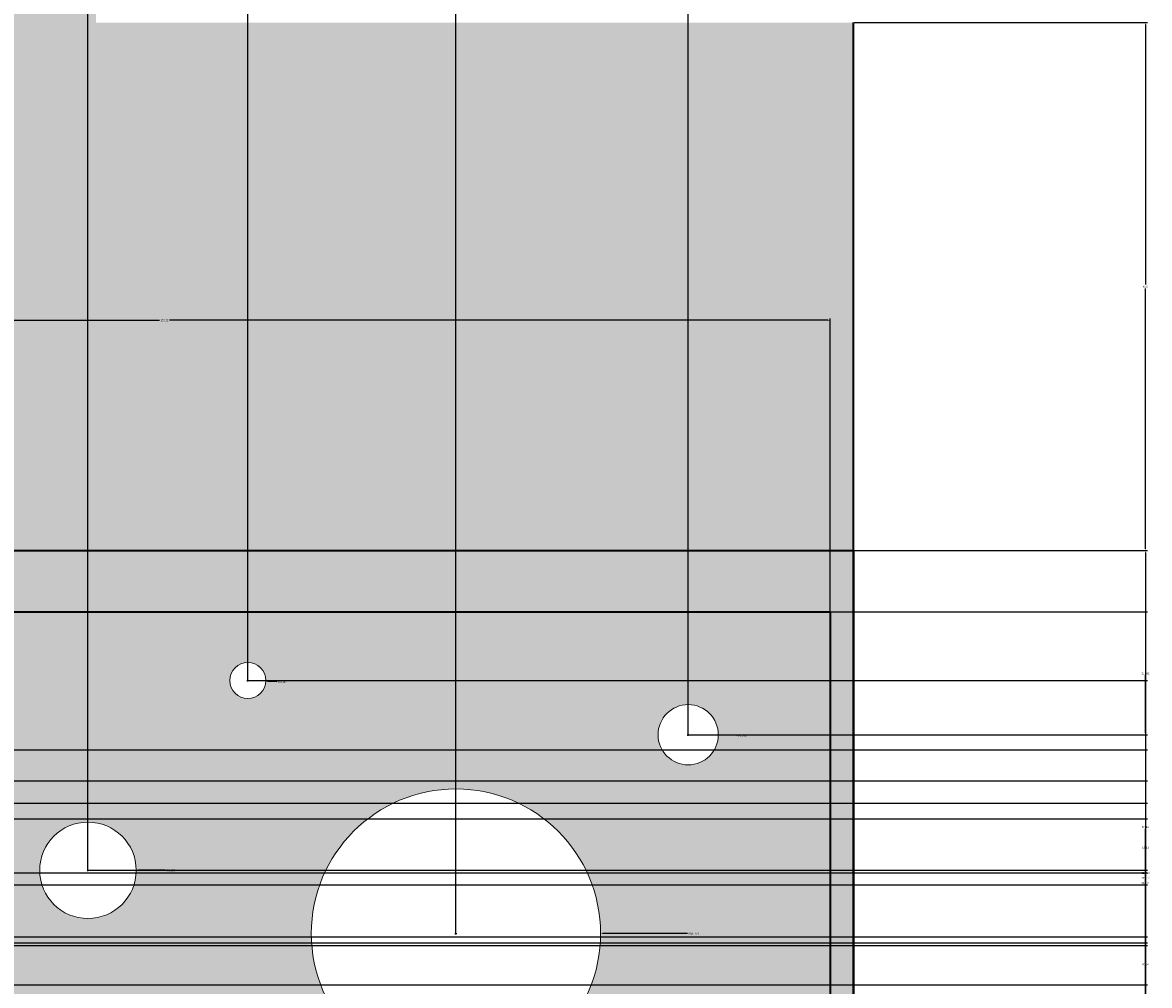
# Model space of a CAD drawing. Units: inches. Extents: x 73 to 607, y 92 to 651.
# Tile 12 of 18: x 503 to 607, y 222 to 311. Entities that reach past the tile are written whole.
import ezdxf

# ---------------------------------------------------------------- set-up
doc = ezdxf.new("R2010")
doc.units = ezdxf.units.IN
doc.header["$MEASUREMENT"] = 0
for name, color, linetype, lineweight in [('A-ANNO-DIMS', 2, 'Continuous', 18), ('A-ELEV', 7, 'Continuous', 35), ('A-ELEV-PANL', 7, 'Continuous', 18), ('A-ELEV-PATT-BKGD', 252, 'Continuous', 13), ('A-ELEV-PATT-SHAD', 8, 'Continuous', 13), ('A-ELEV-PATT-WALL', 254, 'Continuous', 13), ('A-ELEV-PATT-WOOD', 32, 'Continuous', 13)]:
    doc.layers.add(name, color=color, linetype=linetype, lineweight=lineweight)
doc.styles.get("Standard").update_dxf_attribs({"font": 'arial.ttf'})
doc.dimstyles.get("Standard").update_dxf_attribs({"dimtxt": 0.18, "dimasz": 0.18, "dimexe": 0.18, "dimexo": 0.0625, "dimgap": 0.09, "dimtad": 0, "dimtih": 1, "dimtoh": 1, "dimdec": 4, "dimzin": 0, "dimdsep": 46, "dimtxsty": 'Standard', "dimcen": 0.09, "dimadec": 0, "dimazin": 0, "dimtfac": 1, "dimtdec": 4, "dimtofl": 0, "dimtmove": 0, "dimatfit": 3, "dimfxl": 1, "dimtolj": 1, "dimtzin": 0, "dimarcsym": 0})

# ---------------------------------------------------------------- blocks, each defined once
blk = doc.blocks.new('*D17')
at = {"layer": 'A-ANNO-DIMS', "color": 0, "lineweight": -2, "transparency": 16777216}
for p, q in [((580.16, 262.3), (607.28, 262.3)), ((607.1, 262.12), (607.1, 224.16)), ((607.1, 185.84), (607.1, 223.8)), ((431.13, 185.66), (607.28, 185.66))]:
    blk.add_line(p, q, dxfattribs=at)
at = {"layer": 'A-ANNO-DIMS', "color": 0, "transparency": 16777216}
for points in [[(607.07, 262.12), (607.13, 262.12), (607.1, 262.3)], [(607.07, 185.84), (607.13, 185.84), (607.1, 185.66)]]:
    blk.add_solid(points, dxfattribs=at)
at = {"layer": 'Defpoints', "color": 0, "transparency": 16777216}
for p in [(580.1, 262.3), (607.1, 262.3), (431.07, 185.66)]:
    blk.add_point(p, dxfattribs=at)
at = {"layer": 'A-ANNO-DIMS', "color": 0, "transparency": 16777216, "insert": (607.1, 223.98), "char_height": 0.18, "attachment_point": 5}
blk.add_mtext('\\A1;76.64', dxfattribs=at)
blk = doc.blocks.new('*D18')
at = {"layer": 'A-ANNO-DIMS', "color": 0, "lineweight": -2, "transparency": 16777216}
for p, q in [((580.16, 311.2), (607.28, 311.2)), ((607.1, 311.02), (607.1, 286.94)), ((607.1, 262.48), (607.1, 286.57)), ((580.16, 262.3), (607.28, 262.3))]:
    blk.add_line(p, q, dxfattribs=at)
at = {"layer": 'A-ANNO-DIMS', "color": 0, "transparency": 16777216}
for points in [[(607.07, 311.02), (607.13, 311.02), (607.1, 311.2)], [(607.07, 262.48), (607.13, 262.48), (607.1, 262.3)]]:
    blk.add_solid(points, dxfattribs=at)
at = {"layer": 'Defpoints', "color": 0, "transparency": 16777216}
for p in [(580.1, 311.2), (607.1, 311.2), (580.1, 262.3)]:
    blk.add_point(p, dxfattribs=at)
at = {"layer": 'A-ANNO-DIMS', "color": 0, "transparency": 16777216, "insert": (607.1, 286.75), "char_height": 0.18, "attachment_point": 5}
blk.add_mtext('\\A1;48.9', dxfattribs=at)
blk = doc.blocks.new('*D39')
at = {"layer": 'A-ANNO-DIMS', "color": 0, "lineweight": -2, "transparency": 16777216}
for p, q in [((454.7, 256.69), (454.7, 283.81)), ((577.92, 256.69), (577.92, 283.81)), ((454.88, 283.63), (515.86, 283.63)), ((577.74, 283.63), (516.77, 283.63))]:
    blk.add_line(p, q, dxfattribs=at)
at = {"layer": 'A-ANNO-DIMS', "color": 0, "transparency": 16777216}
for points in [[(454.88, 283.66), (454.88, 283.6), (454.7, 283.63)], [(577.74, 283.66), (577.74, 283.6), (577.92, 283.63)]]:
    blk.add_solid(points, dxfattribs=at)
at = {"layer": 'Defpoints', "color": 0, "transparency": 16777216}
for p in [(577.92, 283.63), (454.7, 256.63), (577.92, 256.63)]:
    blk.add_point(p, dxfattribs=at)
at = {"layer": 'A-ANNO-DIMS', "color": 0, "transparency": 16777216, "insert": (516.31, 283.63), "char_height": 0.18, "attachment_point": 5}
blk.add_mtext('\\A1;123.22', dxfattribs=at)
blk = doc.blocks.new('*D61')
at = {"layer": 'A-ANNO-DIMS', "color": 0, "lineweight": -2, "transparency": 16777216}
for p, q in [((543.2, 226.84), (543.38, 226.84)), ((543.29, 226.75), (543.29, 226.93)), ((564.71, 226.84), (556.86, 226.84))]:
    blk.add_line(p, q, dxfattribs=at)
at = {"layer": 'A-ANNO-DIMS', "color": 0, "transparency": 16777216}
blk.add_solid([(556.86, 226.87), (556.86, 226.81), (556.68, 226.84)], dxfattribs=at)
at = {"layer": 'Defpoints', "color": 0, "transparency": 16777216}
for p in [(529.9, 226.84), (556.68, 226.84)]:
    blk.add_point(p, dxfattribs=at)
at = {"layer": 'A-ANNO-DIMS', "color": 0, "transparency": 16777216, "insert": (565.27, 226.84), "char_height": 0.18, "attachment_point": 5}
blk.add_mtext('\\A1;∅26.776', dxfattribs=at)
blk = doc.blocks.new('*D93')
at = {"layer": 'A-ANNO-DIMS', "color": 0, "lineweight": -2, "transparency": 16777216}
for p, q in [((349.06, 237.45), (607.28, 237.45)), ((607.1, 237.27), (607.1, 232.18)), ((607.1, 226.72), (607.1, 231.81)), ((349.06, 226.54), (607.28, 226.54))]:
    blk.add_line(p, q, dxfattribs=at)
at = {"layer": 'A-ANNO-DIMS', "color": 0, "transparency": 16777216}
for points in [[(607.07, 237.27), (607.13, 237.27), (607.1, 237.45)], [(607.07, 226.72), (607.13, 226.72), (607.1, 226.54)]]:
    blk.add_solid(points, dxfattribs=at)
at = {"layer": 'Defpoints', "color": 0, "transparency": 16777216}
for p in [(349, 237.45), (349, 226.54), (607.1, 226.54)]:
    blk.add_point(p, dxfattribs=at)
at = {"layer": 'A-ANNO-DIMS', "color": 0, "transparency": 16777216, "insert": (607.1, 232), "char_height": 0.18, "attachment_point": 5}
blk.add_mtext('\\A1;10.917', dxfattribs=at)
blk = doc.blocks.new('*D95')
at = {"layer": 'A-ANNO-DIMS', "color": 0, "lineweight": -2, "transparency": 16777216}
for p, q in [((363.87, 225.98), (607.28, 225.98)), ((607.1, 225.8), (607.1, 212.75)), ((607.1, 199.33), (607.1, 212.38)), ((363.32, 199.15), (607.28, 199.15))]:
    blk.add_line(p, q, dxfattribs=at)
at = {"layer": 'A-ANNO-DIMS', "color": 0, "transparency": 16777216}
for points in [[(607.07, 225.8), (607.13, 225.8), (607.1, 225.98)], [(607.07, 199.33), (607.13, 199.33), (607.1, 199.15)]]:
    blk.add_solid(points, dxfattribs=at)
at = {"layer": 'Defpoints', "color": 0, "transparency": 16777216}
for p in [(363.81, 225.98), (607.1, 225.98), (363.26, 199.15)]:
    blk.add_point(p, dxfattribs=at)
at = {"layer": 'A-ANNO-DIMS', "color": 0, "transparency": 16777216, "insert": (607.1, 212.57), "char_height": 0.18, "attachment_point": 5}
blk.add_mtext('\\A1;26.83', dxfattribs=at)
blk = doc.blocks.new('*D96')
at = {"layer": 'A-ANNO-DIMS', "color": 0, "lineweight": -2, "transparency": 16777216}
for p, q in [((360.91, 238.93), (607.28, 238.93)), ((607.1, 238.75), (607.1, 232.64)), ((607.1, 226.16), (607.1, 232.28)), ((363.87, 225.98), (607.28, 225.98))]:
    blk.add_line(p, q, dxfattribs=at)
at = {"layer": 'A-ANNO-DIMS', "color": 0, "transparency": 16777216}
for points in [[(607.07, 238.75), (607.13, 238.75), (607.1, 238.93)], [(607.07, 226.16), (607.13, 226.16), (607.1, 225.98)]]:
    blk.add_solid(points, dxfattribs=at)
at = {"layer": 'Defpoints', "color": 0, "transparency": 16777216}
for p in [(360.85, 238.93), (607.1, 238.93), (363.81, 225.98)]:
    blk.add_point(p, dxfattribs=at)
at = {"layer": 'A-ANNO-DIMS', "color": 0, "transparency": 16777216, "insert": (607.1, 232.46), "char_height": 0.18, "attachment_point": 5}
blk.add_mtext('\\A1;12.953', dxfattribs=at)
blk = doc.blocks.new('*D99')
at = {"layer": 'A-ANNO-DIMS', "color": 0, "lineweight": -2, "transparency": 16777216}
for p, q in [((373.32, 231.35), (607.28, 231.35)), ((607.1, 231.17), (607.1, 220.43)), ((607.1, 209.32), (607.1, 220.06)), ((377.02, 209.14), (607.28, 209.14))]:
    blk.add_line(p, q, dxfattribs=at)
at = {"layer": 'A-ANNO-DIMS', "color": 0, "transparency": 16777216}
for points in [[(607.07, 231.17), (607.13, 231.17), (607.1, 231.35)], [(607.07, 209.32), (607.13, 209.32), (607.1, 209.14)]]:
    blk.add_solid(points, dxfattribs=at)
at = {"layer": 'Defpoints', "color": 0, "transparency": 16777216}
for p in [(373.26, 231.35), (607.1, 231.35), (376.96, 209.14)]:
    blk.add_point(p, dxfattribs=at)
at = {"layer": 'A-ANNO-DIMS', "color": 0, "transparency": 16777216, "insert": (607.1, 220.25), "char_height": 0.18, "attachment_point": 5}
blk.add_mtext('\\A1;22.205', dxfattribs=at)
blk = doc.blocks.new('*D100')
at = {"layer": 'A-ANNO-DIMS', "color": 0, "lineweight": -2, "transparency": 16777216}
for p, q in [((382.95, 222.1), (607.28, 222.1)), ((607.1, 221.92), (607.1, 211.27)), ((607.1, 200.26), (607.1, 210.9)), ((387.58, 200.08), (607.28, 200.08))]:
    blk.add_line(p, q, dxfattribs=at)
at = {"layer": 'A-ANNO-DIMS', "color": 0, "transparency": 16777216}
for points in [[(607.07, 221.92), (607.13, 221.92), (607.1, 222.1)], [(607.07, 200.26), (607.13, 200.26), (607.1, 200.08)]]:
    blk.add_solid(points, dxfattribs=at)
at = {"layer": 'Defpoints', "color": 0, "transparency": 16777216}
for p in [(382.89, 222.1), (607.1, 222.1), (387.52, 200.08)]:
    blk.add_point(p, dxfattribs=at)
at = {"layer": 'A-ANNO-DIMS', "color": 0, "transparency": 16777216, "insert": (607.1, 211.09), "char_height": 0.18, "attachment_point": 5}
blk.add_mtext('\\A1;22.02', dxfattribs=at)
blk = doc.blocks.new('*D101')
at = {"layer": 'A-ANNO-DIMS', "color": 0, "lineweight": -2, "transparency": 16777216}
for p, q in [((382.39, 240.97), (607.28, 240.97)), ((607.1, 240.79), (607.1, 231.72)), ((607.1, 222.28), (607.1, 231.35)), ((382.95, 222.1), (607.28, 222.1))]:
    blk.add_line(p, q, dxfattribs=at)
at = {"layer": 'A-ANNO-DIMS', "color": 0, "transparency": 16777216}
for points in [[(607.07, 240.79), (607.13, 240.79), (607.1, 240.97)], [(607.07, 222.28), (607.13, 222.28), (607.1, 222.1)]]:
    blk.add_solid(points, dxfattribs=at)
at = {"layer": 'Defpoints', "color": 0, "transparency": 16777216}
for p in [(382.33, 240.97), (607.1, 240.97), (382.89, 222.1)]:
    blk.add_point(p, dxfattribs=at)
at = {"layer": 'A-ANNO-DIMS', "color": 0, "transparency": 16777216, "insert": (607.1, 231.53), "char_height": 0.18, "attachment_point": 5}
blk.add_mtext('\\A1;18.874', dxfattribs=at)
blk = doc.blocks.new('*D102')
at = {"layer": 'A-ANNO-DIMS', "color": 0, "lineweight": -2, "transparency": 16777216}
for p, q in [((382.39, 240.97), (607.28, 240.97)), ((607.1, 240.79), (607.1, 236.9)), ((607.1, 232.64), (607.1, 236.53)), ((389.62, 232.46), (607.28, 232.46))]:
    blk.add_line(p, q, dxfattribs=at)
at = {"layer": 'A-ANNO-DIMS', "color": 0, "transparency": 16777216}
for points in [[(607.07, 240.79), (607.13, 240.79), (607.1, 240.97)], [(607.07, 232.64), (607.13, 232.64), (607.1, 232.46)]]:
    blk.add_solid(points, dxfattribs=at)
at = {"layer": 'Defpoints', "color": 0, "transparency": 16777216}
for p in [(382.33, 240.97), (389.55, 232.46), (607.1, 232.46)]:
    blk.add_point(p, dxfattribs=at)
at = {"layer": 'A-ANNO-DIMS', "color": 0, "transparency": 16777216, "insert": (607.1, 236.71), "char_height": 0.18, "attachment_point": 5}
blk.add_mtext('\\A1;8.512', dxfattribs=at)
blk = doc.blocks.new('*D106')
at = {"layer": 'A-ANNO-DIMS', "color": 0, "lineweight": -2, "transparency": 16777216}
for p, q in [((482.44, 246.99), (482.44, 650.98)), ((482.62, 650.8), (495.37, 650.8)), ((509.06, 650.8), (496.3, 650.8)), ((509.24, 232.76), (509.24, 650.98))]:
    blk.add_line(p, q, dxfattribs=at)
at = {"layer": 'A-ANNO-DIMS', "color": 0, "transparency": 16777216}
for points in [[(482.62, 650.83), (482.62, 650.77), (482.44, 650.8)], [(509.06, 650.83), (509.06, 650.77), (509.24, 650.8)]]:
    blk.add_solid(points, dxfattribs=at)
at = {"layer": 'Defpoints', "color": 0, "transparency": 16777216}
for p in [(509.24, 650.8), (482.44, 246.92), (509.24, 232.7)]:
    blk.add_point(p, dxfattribs=at)
at = {"layer": 'A-ANNO-DIMS', "color": 0, "transparency": 16777216, "insert": (495.84, 650.8), "char_height": 0.18, "attachment_point": 5}
blk.add_mtext('\\A1;26.797', dxfattribs=at)
blk = doc.blocks.new('*D107')
at = {"layer": 'A-ANNO-DIMS', "color": 0, "lineweight": -2, "transparency": 16777216}
for p, q in [((509.24, 232.76), (509.24, 650.98)), ((509.42, 650.8), (516.18, 650.8)), ((523.85, 650.8), (517.09, 650.8)), ((524.03, 250.33), (524.03, 650.98))]:
    blk.add_line(p, q, dxfattribs=at)
at = {"layer": 'A-ANNO-DIMS', "color": 0, "transparency": 16777216}
for points in [[(509.42, 650.83), (509.42, 650.77), (509.24, 650.8)], [(523.85, 650.83), (523.85, 650.77), (524.03, 650.8)]]:
    blk.add_solid(points, dxfattribs=at)
at = {"layer": 'Defpoints', "color": 0, "transparency": 16777216}
for p in [(524.03, 650.8), (524.03, 250.27), (509.24, 232.7)]:
    blk.add_point(p, dxfattribs=at)
at = {"layer": 'A-ANNO-DIMS', "color": 0, "transparency": 16777216, "insert": (516.63, 650.8), "char_height": 0.18, "attachment_point": 5}
blk.add_mtext('\\A1;14.794', dxfattribs=at)
blk = doc.blocks.new('*D108')
at = {"layer": 'A-ANNO-DIMS', "color": 0, "lineweight": -2, "transparency": 16777216}
for p, q in [((524.03, 250.33), (524.03, 650.98)), ((524.21, 650.8), (533.28, 650.8)), ((543.11, 650.8), (534.05, 650.8)), ((543.29, 226.9), (543.29, 650.98))]:
    blk.add_line(p, q, dxfattribs=at)
at = {"layer": 'A-ANNO-DIMS', "color": 0, "transparency": 16777216}
for points in [[(524.21, 650.83), (524.21, 650.77), (524.03, 650.8)], [(543.11, 650.83), (543.11, 650.77), (543.29, 650.8)]]:
    blk.add_solid(points, dxfattribs=at)
at = {"layer": 'Defpoints', "color": 0, "transparency": 16777216}
for p in [(543.29, 650.8), (524.03, 250.27), (543.29, 226.84)]:
    blk.add_point(p, dxfattribs=at)
at = {"layer": 'A-ANNO-DIMS', "color": 0, "transparency": 16777216, "insert": (533.66, 650.8), "char_height": 0.18, "attachment_point": 5}
blk.add_mtext('\\A1;19.26', dxfattribs=at)
blk = doc.blocks.new('*D109')
at = {"layer": 'A-ANNO-DIMS', "color": 0, "lineweight": -2, "transparency": 16777216}
for p, q in [((543.29, 226.9), (543.29, 650.98)), ((543.47, 650.8), (553.57, 650.8)), ((564.61, 650.8), (554.5, 650.8)), ((564.79, 245.31), (564.79, 650.98))]:
    blk.add_line(p, q, dxfattribs=at)
at = {"layer": 'A-ANNO-DIMS', "color": 0, "transparency": 16777216}
for points in [[(543.47, 650.83), (543.47, 650.77), (543.29, 650.8)], [(564.61, 650.83), (564.61, 650.77), (564.79, 650.8)]]:
    blk.add_solid(points, dxfattribs=at)
at = {"layer": 'Defpoints', "color": 0, "transparency": 16777216}
for p in [(564.79, 650.8), (564.79, 245.25), (543.29, 226.84)]:
    blk.add_point(p, dxfattribs=at)
at = {"layer": 'A-ANNO-DIMS', "color": 0, "transparency": 16777216, "insert": (554.04, 650.8), "char_height": 0.18, "attachment_point": 5}
blk.add_mtext('\\A1;21.493', dxfattribs=at)
blk = doc.blocks.new('*D120')
at = {"layer": 'A-ANNO-DIMS', "color": 0, "lineweight": -2, "transparency": 16777216}
for p, q in [((468.55, 225.73), (607.28, 225.73)), ((607.1, 225.55), (607.1, 208.62)), ((607.1, 191.32), (607.1, 208.25)), ((469.94, 191.14), (607.28, 191.14))]:
    blk.add_line(p, q, dxfattribs=at)
at = {"layer": 'A-ANNO-DIMS', "color": 0, "transparency": 16777216}
for points in [[(607.07, 225.55), (607.13, 225.55), (607.1, 225.73)], [(607.07, 191.32), (607.13, 191.32), (607.1, 191.14)]]:
    blk.add_solid(points, dxfattribs=at)
at = {"layer": 'Defpoints', "color": 0, "transparency": 16777216}
for p in [(468.48, 225.73), (607.1, 225.73), (469.88, 191.14)]:
    blk.add_point(p, dxfattribs=at)
at = {"layer": 'A-ANNO-DIMS', "color": 0, "transparency": 16777216, "insert": (607.1, 208.43), "char_height": 0.18, "attachment_point": 5}
blk.add_mtext('\\A1;34.585', dxfattribs=at)
blk = doc.blocks.new('*D121')
at = {"layer": 'A-ANNO-DIMS', "color": 0, "lineweight": -2, "transparency": 16777216}
for p, q in [((463.24, 243.86), (607.28, 243.86)), ((607.1, 243.68), (607.1, 234.97)), ((607.1, 225.91), (607.1, 234.61)), ((468.55, 225.73), (607.28, 225.73))]:
    blk.add_line(p, q, dxfattribs=at)
at = {"layer": 'A-ANNO-DIMS', "color": 0, "transparency": 16777216}
for points in [[(607.07, 243.68), (607.13, 243.68), (607.1, 243.86)], [(607.07, 225.91), (607.13, 225.91), (607.1, 225.73)]]:
    blk.add_solid(points, dxfattribs=at)
at = {"layer": 'Defpoints', "color": 0, "transparency": 16777216}
for p in [(463.18, 243.86), (607.1, 243.86), (468.48, 225.73)]:
    blk.add_point(p, dxfattribs=at)
at = {"layer": 'A-ANNO-DIMS', "color": 0, "transparency": 16777216, "insert": (607.1, 234.79), "char_height": 0.18, "attachment_point": 5}
blk.add_mtext('\\A1;18.13', dxfattribs=at)
blk = doc.blocks.new('*D126')
at = {"layer": 'A-ANNO-DIMS', "color": 0, "lineweight": -2, "transparency": 16777216}
for p, q in [((509.3, 232.7), (607.28, 232.7)), ((607.1, 232.52), (607.1, 213.92)), ((607.1, 194.95), (607.1, 213.55)), ((509.02, 194.77), (607.28, 194.77))]:
    blk.add_line(p, q, dxfattribs=at)
at = {"layer": 'A-ANNO-DIMS', "color": 0, "transparency": 16777216}
for points in [[(607.07, 232.52), (607.13, 232.52), (607.1, 232.7)], [(607.07, 194.95), (607.13, 194.95), (607.1, 194.77)]]:
    blk.add_solid(points, dxfattribs=at)
at = {"layer": 'Defpoints', "color": 0, "transparency": 16777216}
for p in [(509.24, 232.7), (607.1, 232.7), (508.96, 194.77)]:
    blk.add_point(p, dxfattribs=at)
at = {"layer": 'A-ANNO-DIMS', "color": 0, "transparency": 16777216, "insert": (607.1, 213.73), "char_height": 0.18, "attachment_point": 5}
blk.add_mtext('\\A1;37.93', dxfattribs=at)
blk = doc.blocks.new('*D127')
at = {"layer": 'A-ANNO-DIMS', "color": 0, "lineweight": -2, "transparency": 16777216}
for p, q in [((524.09, 250.27), (607.28, 250.27)), ((607.1, 250.09), (607.1, 218.66)), ((607.1, 186.86), (607.1, 218.29)), ((523.82, 186.68), (607.28, 186.68))]:
    blk.add_line(p, q, dxfattribs=at)
at = {"layer": 'A-ANNO-DIMS', "color": 0, "transparency": 16777216}
for points in [[(607.07, 250.09), (607.13, 250.09), (607.1, 250.27)], [(607.07, 186.86), (607.13, 186.86), (607.1, 186.68)]]:
    blk.add_solid(points, dxfattribs=at)
at = {"layer": 'Defpoints', "color": 0, "transparency": 16777216}
for p in [(524.03, 250.27), (607.1, 250.27), (523.75, 186.68)]:
    blk.add_point(p, dxfattribs=at)
at = {"layer": 'A-ANNO-DIMS', "color": 0, "transparency": 16777216, "insert": (607.1, 218.47), "char_height": 0.18, "attachment_point": 5}
blk.add_mtext('\\A1;63.59', dxfattribs=at)
blk = doc.blocks.new('*D131')
at = {"layer": 'A-ANNO-DIMS', "color": 0, "lineweight": -2, "transparency": 16777216}
for p, q in [((577.99, 256.63), (607.28, 256.63)), ((607.1, 256.45), (607.1, 251.12)), ((607.1, 245.43), (607.1, 250.76)), ((564.85, 245.25), (607.28, 245.25))]:
    blk.add_line(p, q, dxfattribs=at)
at = {"layer": 'A-ANNO-DIMS', "color": 0, "transparency": 16777216}
for points in [[(607.07, 256.45), (607.13, 256.45), (607.1, 256.63)], [(607.07, 245.43), (607.13, 245.43), (607.1, 245.25)]]:
    blk.add_solid(points, dxfattribs=at)
at = {"layer": 'Defpoints', "color": 0, "transparency": 16777216}
for p in [(577.92, 256.63), (564.79, 245.25), (607.1, 245.25)]:
    blk.add_point(p, dxfattribs=at)
at = {"layer": 'A-ANNO-DIMS', "color": 0, "transparency": 16777216, "insert": (607.1, 250.94), "char_height": 0.18, "attachment_point": 5}
blk.add_mtext('\\A1;11.382', dxfattribs=at)
blk = doc.blocks.new('*D156')
at = {"layer": 'A-ANNO-DIMS', "color": 0, "lineweight": -2, "transparency": 16777216}
for p, q in [((524.03, 250.18), (524.03, 250.36)), ((523.94, 250.27), (524.12, 250.27)), ((526.71, 250.16), (525.88, 250.19))]:
    blk.add_line(p, q, dxfattribs=at)
at = {"layer": 'A-ANNO-DIMS', "color": 0, "transparency": 16777216}
blk.add_solid([(525.88, 250.22), (525.88, 250.16), (525.7, 250.2)], dxfattribs=at)
at = {"layer": 'Defpoints', "color": 0, "transparency": 16777216}
for p in [(522.36, 250.34), (525.7, 250.2)]:
    blk.add_point(p, dxfattribs=at)
at = {"layer": 'A-ANNO-DIMS', "color": 0, "transparency": 16777216, "insert": (527.2, 250.16), "char_height": 0.18, "attachment_point": 5}
blk.add_mtext('\\A1;∅3.347', dxfattribs=at)
blk = doc.blocks.new('*D157')
at = {"layer": 'A-ANNO-DIMS', "color": 0, "lineweight": -2, "transparency": 16777216}
for p, q in [((564.7, 245.25), (564.88, 245.25)), ((564.79, 245.16), (564.79, 245.34)), ((569.25, 245.17), (567.75, 245.2))]:
    blk.add_line(p, q, dxfattribs=at)
at = {"layer": 'A-ANNO-DIMS', "color": 0, "transparency": 16777216}
blk.add_solid([(567.75, 245.23), (567.75, 245.17), (567.57, 245.2)], dxfattribs=at)
at = {"layer": 'Defpoints', "color": 0, "transparency": 16777216}
for p in [(562, 245.3), (567.57, 245.2)]:
    blk.add_point(p, dxfattribs=at)
at = {"layer": 'A-ANNO-DIMS', "color": 0, "transparency": 16777216, "insert": (569.74, 245.17), "char_height": 0.18, "attachment_point": 5}
blk.add_mtext('\\A1;∅5.578', dxfattribs=at)
blk = doc.blocks.new('*D158')
at = {"layer": 'A-ANNO-DIMS', "color": 0, "lineweight": -2, "transparency": 16777216}
for p, q in [((509.15, 232.7), (509.33, 232.7)), ((509.24, 232.61), (509.24, 232.79)), ((516.38, 232.7), (513.88, 232.7))]:
    blk.add_line(p, q, dxfattribs=at)
at = {"layer": 'A-ANNO-DIMS', "color": 0, "transparency": 16777216}
blk.add_solid([(513.88, 232.73), (513.88, 232.67), (513.7, 232.7)], dxfattribs=at)
at = {"layer": 'Defpoints', "color": 0, "transparency": 16777216}
for p in [(504.78, 232.7), (513.7, 232.7)]:
    blk.add_point(p, dxfattribs=at)
at = {"layer": 'A-ANNO-DIMS', "color": 0, "transparency": 16777216, "insert": (516.87, 232.7), "char_height": 0.18, "attachment_point": 5}
blk.add_mtext('\\A1;∅8.925', dxfattribs=at)
blk = doc.blocks.new('*D159')
at = {"layer": 'A-ANNO-DIMS', "color": 0, "lineweight": -2, "transparency": 16777216}
for p, q in [((543.2, 226.84), (543.38, 226.84)), ((543.29, 226.75), (543.29, 226.93)), ((543.29, 205.42), (543.29, 213.27)), ((543.11, 205.42), (543.29, 205.42))]:
    blk.add_line(p, q, dxfattribs=at)
at = {"layer": 'A-ANNO-DIMS', "color": 0, "transparency": 16777216}
blk.add_solid([(543.26, 213.27), (543.32, 213.27), (543.29, 213.45)], dxfattribs=at)
at = {"layer": 'Defpoints', "color": 0, "transparency": 16777216}
for p in [(543.29, 240.23), (543.29, 213.45)]:
    blk.add_point(p, dxfattribs=at)
at = {"layer": 'A-ANNO-DIMS', "color": 0, "transparency": 16777216, "insert": (542.55, 205.42), "char_height": 0.18, "attachment_point": 5}
blk.add_mtext('\\A1;∅26.776', dxfattribs=at)

msp = doc.modelspace()

# ---------------------------------------------------------------- hatches: boundary and pattern name
at = {"layer": 'A-ELEV-PATT-BKGD'}
h = msp.add_hatch(color=256, dxfattribs=at)
h.dxf.hatch_style = 1
h.paths.add_polyline_path([(321.3008, 479.2042), (312.3008, 479.2042), (312.3008, 478.7576), (312.3008, 412.636), (321.3008, 412.636)])
h.paths.add_polyline_path([(312.3008, 504.7576), (256.4726, 504.7576), (256.4726, 503.4576), (312.3008, 503.4576)], flags=17)
h.paths.add_polyline_path([(321.3008, 543.1576), (321.3008, 552.1576), (320.3257, 552.1576), (312.3008, 552.1576), (256.4726, 552.1576), (256.4726, 543.1576), (312.3008, 543.1576), (312.3008, 479.2042), (321.3008, 479.2042)])
h.paths.add_polyline_path([(451.5214, 412.636), (256.4726, 412.636), (256.4726, 403.636), (442.5214, 403.636), (442.5214, 320.2042), (206.1343, 320.2042), (206.1343, 320.9135), (206.1343, 403.636), (256.4726, 403.636), (256.4726, 412.636), (201.6343, 412.636), (201.6343, 320.9135), (201.6343, 320.2042), (201.6343, 311.2042), (256.4726, 311.2042), (451.5214, 311.2042)])
h.paths.add_polyline_path([(431.07, 258.6914), (369.5339, 258.6914), (369.5339, 247.4054), (396.692, 247.4054), (425.07, 247.4054), (425.07, 194.7312), (396.692, 194.6197), (396.692, 194.5366), (369.5339, 194.5366), (369.5339, 185.6619), (431.07, 185.6619)])
h.paths.add_polyline_path([(580.0983, 262.3024), (451.5214, 262.3024), (451.5214, 143.2042), (580.0983, 143.2042)])
h.paths.add_polyline_path([(454.7049, 174.802), (454.7049, 256.6321), (577.9249, 256.6321), (577.9249, 174.802)], flags=16)
h.paths.add_polyline_path([(465.9716, 191.1416, -1), (473.7874, 191.1416, -1)], flags=0)
h.paths.add_polyline_path([(490.5373, 181.6586, -1), (494.9999, 181.6586, -1)], flags=0)
h.paths.add_polyline_path([(476.2996, 209.8287, -1), (500.5844, 209.8287, -1)], flags=0)
h.paths.add_polyline_path([(505.3326, 194.7675, -1), (512.5843, 194.7675, -1)], flags=0)
h.paths.add_polyline_path([(520.9613, 186.679, -1), (526.544, 186.679, -1)], flags=0)
h.paths.add_polyline_path([(466.8103, 225.7267, -1), (470.1573, 225.7267, -1)], flags=0)
h.paths.add_polyline_path([(527.1059, 203.6926, -1), (536.0311, 203.6926, -1)], flags=0)
h.paths.add_polyline_path([(504.775, 232.6995, -1), (513.7002, 232.6995, -1)], flags=0)
h.paths.add_polyline_path([(546.9241, 183.611, -1), (554.7336, 183.611, -1)], flags=0)
h.paths.add_polyline_path([(459.5544, 243.856, -1), (466.8061, 243.856, -1)], flags=0)
h.paths.add_polyline_path([(476.3045, 246.924, -1), (488.5767, 246.924, -1)], flags=0)
h.paths.add_polyline_path([(529.9044, 226.8424, -1), (556.68, 226.8424, -1)], flags=0)
h.paths.add_polyline_path([(554.1814, 203.9716, -1), (561.4331, 203.9716, -1)], flags=0)
h.paths.add_polyline_path([(567.8561, 193.3729, -1), (570.6475, 193.3729, -1)], flags=0)
h.paths.add_polyline_path([(522.3584, 250.271, -1), (525.7053, 250.271, -1)], flags=0)
h.paths.add_polyline_path([(561.9965, 245.2506, -1), (567.5748, 245.2506, -1)], flags=0)
h.paths.add_polyline_path([(347.8686, 194.5366), (341.8686, 194.5366), (341.8686, 194.5452), (314.0144, 194.5452), (314.0144, 188.5452), (347.8686, 188.5452)])
h.paths.add_polyline_path([(347.8686, 253.4054), (314.0144, 253.4054), (314.0144, 247.4054), (341.8686, 247.4054), (347.8686, 247.4054)])
h.paths.add_polyline_path([(304.3559, 253.4054), (298.3559, 253.4054), (298.3559, 188.5452), (304.3559, 188.5452)])
h.paths.add_polyline_path([(450.6603, 552.1576), (369.9727, 552.1576), (369.9727, 479.2042), (374.4727, 479.2042), (374.4727, 547.6576), (446.1603, 547.6576), (446.1603, 479.2042), (450.6603, 479.2042)])
h.paths.add_polyline_path([(374.4727, 479.2042), (369.9727, 479.2042), (369.9727, 465.0632), (374.4727, 465.0632)])
h.paths.add_polyline_path([(450.6603, 479.2042), (446.1603, 479.2042), (446.1603, 465.0632), (450.6603, 465.0632)])
h.paths.add_polyline_path([(256.4726, 281.6039), (109.0983, 281.6039), (100.0983, 281.6039), (100.0983, 167.2042), (100.0983, 143.2042), (109.0983, 143.2042), (109.0983, 167.2042), (109.0983, 272.6039), (256.4726, 272.6039)])
at = {"layer": 'A-ELEV-PATT-SHAD'}
h = msp.add_hatch(color=256, dxfattribs=at)
h.dxf.hatch_style = 1
h.paths.add_polyline_path([(451.5214, 412.636), (256.4726, 412.636), (256.4726, 403.636), (442.5214, 403.636), (442.5214, 320.2042), (206.1343, 320.2042), (206.1343, 320.9135), (206.1343, 403.636), (256.4726, 403.636), (256.4726, 412.636), (201.6343, 412.636), (201.6343, 320.9135), (201.6343, 320.2042), (201.6343, 311.2042), (256.4726, 311.2042), (451.5214, 311.2042)])
h.paths.add_polyline_path([(580.0983, 262.3024), (451.5214, 262.3024), (451.5214, 143.2042), (580.0983, 143.2042)])
h.paths.add_polyline_path([(454.7049, 174.802), (454.7049, 256.6321), (577.9249, 256.6321), (577.9249, 174.802)], flags=16)
h.paths.add_polyline_path([(465.9716, 191.1416, -1), (473.7874, 191.1416, -1)], flags=0)
h.paths.add_polyline_path([(490.5373, 181.6586, -1), (494.9999, 181.6586, -1)], flags=0)
h.paths.add_polyline_path([(476.2996, 209.8287, -1), (500.5844, 209.8287, -1)], flags=0)
h.paths.add_polyline_path([(505.3326, 194.7675, -1), (512.5843, 194.7675, -1)], flags=0)
h.paths.add_polyline_path([(520.9613, 186.679, -1), (526.544, 186.679, -1)], flags=0)
h.paths.add_polyline_path([(466.8103, 225.7267, -1), (470.1573, 225.7267, -1)], flags=0)
h.paths.add_polyline_path([(527.1059, 203.6926, -1), (536.0311, 203.6926, -1)], flags=0)
h.paths.add_polyline_path([(459.5544, 243.856, -1), (466.8061, 243.856, -1)], flags=0)
h.paths.add_polyline_path([(504.775, 232.6995, -1), (513.7002, 232.6995, -1)], flags=0)
h.paths.add_polyline_path([(476.3045, 246.924, -1), (488.5767, 246.924, -1)], flags=0)
h.paths.add_polyline_path([(546.9241, 183.611, -1), (554.7336, 183.611, -1)], flags=0)
h.paths.add_polyline_path([(529.9044, 226.8424, -1), (556.68, 226.8424, -1)], flags=0)
h.paths.add_polyline_path([(554.1814, 203.9716, -1), (561.4331, 203.9716, -1)], flags=0)
h.paths.add_polyline_path([(522.3584, 250.271, -1), (525.7053, 250.271, -1)], flags=0)
h.paths.add_polyline_path([(567.8561, 193.3729, -1), (570.6475, 193.3729, -1)], flags=0)
h.paths.add_polyline_path([(561.9965, 245.2506, -1), (567.5748, 245.2506, -1)], flags=0)
h.paths.add_polyline_path([(431.07, 258.6914), (369.5339, 258.6914), (369.5339, 247.4054), (396.692, 247.4054), (425.07, 247.4054), (425.07, 194.7312), (396.692, 194.6197), (396.692, 194.5366), (369.5339, 194.5366), (369.5339, 185.6619), (431.07, 185.6619)])
h.paths.add_polyline_path([(347.8686, 253.4054), (314.0144, 253.4054), (314.0144, 247.4054), (341.8686, 247.4054), (347.8686, 247.4054)])
h.paths.add_polyline_path([(304.3559, 253.4054), (298.3559, 253.4054), (298.3559, 188.5452), (304.3559, 188.5452)])
h.paths.add_polyline_path([(347.8686, 194.5366), (341.8686, 194.5366), (341.8686, 194.5452), (314.0144, 194.5452), (314.0144, 188.5452), (347.8686, 188.5452)])
at = {"layer": 'A-ELEV-PATT-WALL'}
h = msp.add_hatch(color=256, dxfattribs=at)
h.dxf.hatch_style = 1
h.paths.add_polyline_path([(509.9692, 483.857), (450.6603, 483.857), (450.6603, 465.0632), (446.1603, 465.0632), (446.1603, 484.2142), (374.4727, 484.2142), (374.4727, 465.0632), (369.9727, 465.0632), (369.9727, 484.2142), (321.3008, 484.2142), (321.3008, 412.636), (451.5214, 412.636), (451.5214, 311.2042), (314.0144, 311.2042), (314.0144, 253.4054), (347.8686, 253.4054), (347.8686, 247.4054), (369.5339, 247.4054), (369.5339, 258.6914), (431.07, 258.6914), (431.07, 185.6619), (369.5339, 185.6619), (369.5339, 194.5366), (347.8686, 194.5366), (347.8686, 188.5452), (314.0144, 188.5452), (314.0144, 143.2042), (451.5214, 143.2042), (451.5214, 262.3024), (580.0983, 262.3024), (580.0983, 311.2042), (509.9692, 311.2042)])
h.paths.add_polyline_path([(304.3559, 311.2042), (256.4726, 311.2042), (256.4726, 167.2042), (256.4726, 143.2042), (304.3559, 143.2042), (304.3559, 188.5452), (298.3559, 188.5452), (298.3559, 253.4054), (304.3559, 253.4054)])
at = {"layer": 'A-ELEV-PATT-WOOD'}
h = msp.add_hatch(color=256, dxfattribs=at)
h.dxf.hatch_style = 1
h.paths.add_polyline_path([(577.9249, 256.6321), (454.7049, 256.6321), (454.7049, 174.802), (577.9249, 174.802)])
h.paths.add_polyline_path([(476.2996, 209.8287, -1), (500.5844, 209.8287, -1)], flags=16)
h.paths.add_polyline_path([(473.7874, 191.1416, -1), (465.9716, 191.1416, -1)], flags=16)
h.paths.add_polyline_path([(466.8103, 225.7267, -1), (470.1573, 225.7267, -1)], flags=16)
h.paths.add_polyline_path([(459.5544, 243.856, -1), (466.8061, 243.856, -1)], flags=16)
h.paths.add_polyline_path([(494.9999, 181.6586, -1), (490.5373, 181.6586, -1)], flags=16)
h.paths.add_polyline_path([(476.3045, 246.924, -1), (488.5767, 246.924, -1)], flags=16)
h.paths.add_polyline_path([(512.5843, 194.7675, -1), (505.3326, 194.7675, -1)], flags=16)
h.paths.add_polyline_path([(504.775, 232.6995, -1), (513.7002, 232.6995, -1)], flags=16)
h.paths.add_polyline_path([(526.544, 186.679, -1), (520.9613, 186.679, -1)], flags=16)
h.paths.add_polyline_path([(536.0311, 203.6926, -1), (527.1059, 203.6926, -1)], flags=16)
h.paths.add_polyline_path([(529.9044, 226.8424, -1), (556.68, 226.8424, -1)], flags=16)
h.paths.add_polyline_path([(522.3584, 250.271, -1), (525.7053, 250.271, -1)], flags=16)
h.paths.add_polyline_path([(554.7336, 183.611, -1), (546.9241, 183.611, -1)], flags=16)
h.paths.add_polyline_path([(561.4331, 203.9716, -1), (554.1814, 203.9716, -1)], flags=16)
h.paths.add_polyline_path([(561.9965, 245.2506, -1), (567.5748, 245.2506, -1)], flags=16)
h.paths.add_polyline_path([(570.6475, 193.3729, -1), (567.8561, 193.3729, -1)], flags=16)

# ---------------------------------------------------------------- linework, layer by layer
at = {"layer": 'A-ELEV'}
msp.add_line((580.0983, 167.2042), (580.0983, 311.2042), dxfattribs=at)
for points in [[(580.0983, 143.2042), (451.5214, 143.2042), (451.5214, 262.3024), (580.0983, 262.3024)], [(454.7049, 256.6321), (577.9249, 256.6321), (577.9249, 174.802), (454.7049, 174.802)]]:
    msp.add_lwpolyline(points, close=True, dxfattribs=at)
at = {"layer": 'A-ELEV-PANL'}
for centre, radius in [((524.0318, 250.271), 1.6735), ((564.7856, 245.2506), 2.7891), ((543.2922, 226.8424), 13.3878), ((509.2376, 232.6995), 4.4626)]:
    msp.add_circle(centre, radius, dxfattribs=at)

# ---------------------------------------------------------------- dimensions: what is measured, and where the dimension line sits
at = {"layer": 'A-ANNO-DIMS'}
for base, p1, p2, override, picture, middle in [((509.2376, 650.801), (482.4406, 246.924), (509.2376, 232.6995), {"dimdec": 3, "dimlfac": 1, "dimrnd": 0, "dimzin": 0, "dimdsep": 46, "dimlunit": 2}, '*D106', (495.8391, 650.801)), ((524.0318, 650.801), (509.2376, 232.6995), (524.0318, 250.271), {"dimdec": 3, "dimlfac": 1, "dimrnd": 0, "dimzin": 0, "dimdsep": 46, "dimlunit": 2}, '*D107', (516.6347, 650.801)), ((543.2922, 650.801), (524.0318, 250.271), (543.2922, 226.8424), {"dimdec": 2, "dimlfac": 1, "dimrnd": 0, "dimzin": 0, "dimdsep": 46, "dimlunit": 2}, '*D108', (533.662, 650.801)), ((564.7856, 650.801), (543.2922, 226.8424), (564.7856, 245.2506), {"dimdec": 3, "dimlfac": 1, "dimrnd": 0, "dimzin": 0, "dimdsep": 46, "dimlunit": 2}, '*D109', (554.0389, 650.801)), ((577.9249, 283.6321), (454.7049, 256.6321), (577.9249, 256.6321), {"dimdec": 2, "dimlfac": 1, "dimrnd": 0, "dimzin": 0, "dimdsep": 46, "dimlunit": 2}, '*D39', (516.3149, 283.6321))]:
    dim = msp.add_linear_dim(base=base, p1=p1, p2=p2, dimstyle='Standard', override=override, dxfattribs=at)
    dim.commit()
    dim.dimension.update_dxf_attribs({"geometry": picture, "text_midpoint": middle})
for base, p1, p2, override, picture, middle in [((607.0983, 311.2042), (580.0983, 262.3024), (580.0983, 311.2042), {"dimdec": 1, "dimlfac": 1, "dimrnd": 0, "dimzin": 0, "dimdsep": 46, "dimlunit": 2}, '*D18', (607.0983, 286.7533)), ((607.0983, 262.3024), (431.07, 185.6619), (580.0983, 262.3024), {"dimdec": 2, "dimlfac": 1, "dimrnd": 0, "dimzin": 0, "dimdsep": 46, "dimlunit": 2}, '*D17', (607.0983, 223.9821)), ((607.0983, 245.25056), (577.92487, 256.63214), (564.78565, 245.25056), {"dimdec": 3, "dimlfac": 1, "dimrnd": 0, "dimzin": 0, "dimdsep": 46, "dimlunit": 2}, '*D131', (607.0983, 250.94135)), ((607.0983, 250.271), (523.7527, 186.679), (524.0318, 250.271), {"dimdec": 2, "dimlfac": 1, "dimrnd": 0, "dimzin": 0, "dimdsep": 46, "dimlunit": 2}, '*D127', (607.0983, 218.475)), ((607.0983, 243.856), (468.4838, 225.7267), (463.1802, 243.856), {"dimdec": 2, "dimlfac": 1, "dimrnd": 0, "dimzin": 0, "dimdsep": 46, "dimlunit": 2}, '*D121', (607.0983, 234.7914)), ((607.0983, 240.9703), (382.8864, 222.0962), (382.3308, 240.9703), {"dimdec": 3, "dimlfac": 1, "dimrnd": 0, "dimzin": 0, "dimdsep": 46, "dimlunit": 2}, '*D101', (607.0983, 231.5333)), ((607.0983, 232.4585), (382.3308, 240.9703), (389.5532, 232.4585), {"dimdec": 3, "dimlfac": 1, "dimrnd": 0, "dimzin": 0, "dimdsep": 46, "dimlunit": 2}, '*D102', (607.0983, 236.7144)), ((607.0983, 238.9349), (363.8119, 225.982), (360.8489, 238.9349), {"dimdec": 3, "dimlfac": 1, "dimrnd": 0, "dimzin": 0, "dimdsep": 46, "dimlunit": 2}, '*D96', (607.0983, 232.4585)), ((607.0983, 226.5372), (348.9968, 237.4546), (348.9968, 226.5372), {"dimdec": 3, "dimlfac": 1, "dimrnd": 0, "dimzin": 0, "dimdsep": 46, "dimlunit": 2}, '*D93', (607.0983, 231.9959)), ((607.0983, 232.6995), (508.9585, 194.7675), (509.2376, 232.6995), {"dimdec": 2, "dimlfac": 1, "dimrnd": 0, "dimzin": 0, "dimdsep": 46, "dimlunit": 2}, '*D126', (607.0983, 213.7335)), ((607.0983, 231.3482), (376.9603, 209.1433), (373.2566, 231.3482), {"dimdec": 3, "dimlfac": 1, "dimrnd": 0, "dimzin": 0, "dimdsep": 46, "dimlunit": 2}, '*D99', (607.0983, 220.2458)), ((607.0983, 225.982), (363.2564, 199.1512), (363.8119, 225.982), {"dimdec": 2, "dimlfac": 1, "dimrnd": 0, "dimzin": 0, "dimdsep": 46, "dimlunit": 2}, '*D95', (607.0983, 212.5666)), ((607.0983, 225.7267), (469.8795, 191.1416), (468.4838, 225.7267), {"dimdec": 3, "dimlfac": 1, "dimrnd": 0, "dimzin": 0, "dimdsep": 46, "dimlunit": 2}, '*D120', (607.0983, 208.4342)), ((607.0983, 222.0962), (387.5161, 200.0764), (382.8864, 222.0962), {"dimdec": 2, "dimlfac": 1, "dimrnd": 0, "dimzin": 0, "dimdsep": 46, "dimlunit": 2}, '*D100', (607.0983, 211.0863))]:
    dim = msp.add_linear_dim(base=base, p1=p1, p2=p2, angle=90, dimstyle='Standard', override=override, dxfattribs=at)
    dim.commit()
    dim.dimension.update_dxf_attribs({"geometry": picture, "text_midpoint": middle})
for p1, p2, picture, middle in [((522.3598, 250.3404), (525.7039, 250.2015), '*D156', (526.7071, 250.1598)), ((561.9969, 245.2988), (567.5744, 245.2023), '*D157', (569.2476, 245.1734)), ((543.2944, 240.2301), (543.29, 213.4546), '*D159', (542.5472, 205.4219)), ((504.775, 232.699), (513.7002, 232.7), '*D158', (516.3778, 232.7003)), ((529.9044, 226.8427), (556.68, 226.842), '*D61', (564.7126, 226.8418))]:
    dim = msp.add_diameter_dim_2p(p1=p1, p2=p2, dimstyle='Standard', override={"dimdec": 3, "dimlfac": 1, "dimrnd": 0, "dimzin": 0, "dimdsep": 46, "dimlunit": 2}, dxfattribs=at)
    dim.commit()
    dim.dimension.update_dxf_attribs({"geometry": picture, "text_midpoint": middle, "dimtype": 163})

doc.saveas('drawing.dxf')
